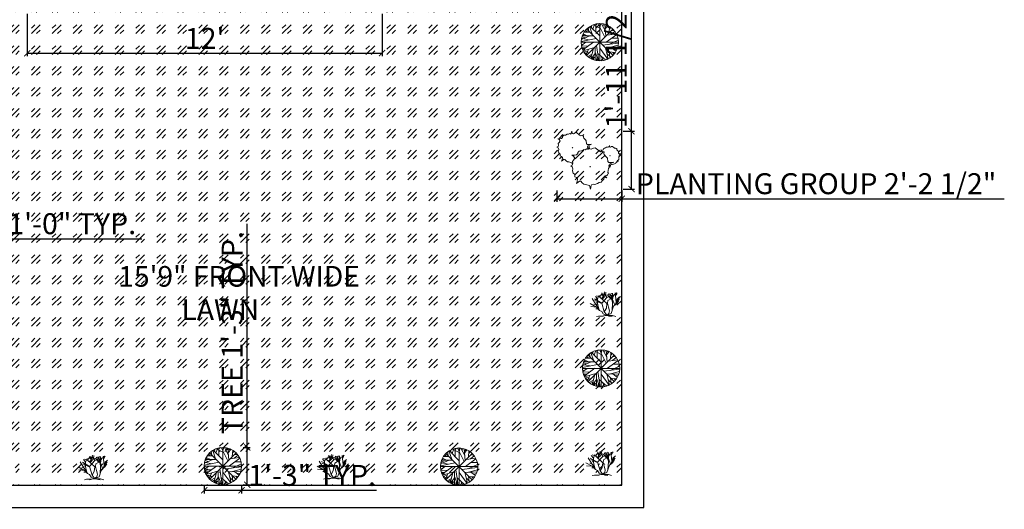
# Model space of a CAD drawing. Units: inches. Extents: x 3799 to 20199, y 1682 to 8087.
# Tile 8 of 30: x 11366 to 11765, y 2123 to 2322. Entities that reach past the tile are written whole.
import ezdxf

# ---------------------------------------------------------------- set-up
doc = ezdxf.new("R2010")
doc.units = ezdxf.units.IN
for name, color, linetype, lineweight in [('A-ANNO-DIMS', 2, 'Continuous', 18), ('A-ANNO-TEXT', 7, 'Continuous', 18), ('A-AREA-IDEN', 7, 'Continuous', 18), ('C-PROP', 7, 'Continuous', 25), ('L-PLNT', 94, 'Continuous', 13), ('L-PLNT-PATT', 94, 'Continuous', 13)]:
    doc.layers.add(name, color=color, linetype=linetype, lineweight=lineweight)
doc.styles.get("Standard").update_dxf_attribs({"font": 'arial.ttf'})
doc.dimstyles.new('ISO-25', dxfattribs={"dimtxt": 8.5, "dimasz": 2.5, "dimexe": 1.25, "dimexo": 0.625, "dimtad": 1, "dimdec": 0, "dimlunit": 3, "dimtxsty": 'Standard', "dimblk": 'ARCHTICK', "dimcen": 2.5, "dimadec": 0, "dimazin": 0, "dimtfac": 1, "dimtdec": 0, "dimtmove": 0, "dimatfit": 3, "dimfxl": 1, "dimarcsym": 0})

# ---------------------------------------------------------------- blocks, each defined once
blk = doc.blocks.new('Clump of Trees or Bushes - plan')
for points in [[(-10.993, 56.487), (-9.228, 58.426), (-10.144, 63.512), (-8.923, 67.033), (-3.43, 69.772), (2.673, 72.119), (-2.82, 71.728), (-10.449, 71.728), (-13.195, 74.075), (-13.806, 83.073), (-16.857, 86.594), (-22.045, 92.071), (-22.961, 94.81), (-22.656, 98.722), (-28.759, 100.678), (-31.811, 99.113), (-35.472, 101.461), (-45.543, 109.676), (-49.815, 108.503), (-55.308, 106.155), (-59.58, 106.938), (-60.801, 113.98), (-63.242, 104.982), (-67.209, 106.938), (-70.872, 104.59), (-74.839, 104.982), (-80.637, 101.461), (-86.435, 101.069), (-90.402, 97.548), (-90.402, 94.419), (-93.454, 90.898), (-98.947, 90.115), (-105.66, 90.115), (-101.083, 87.768), (-98.031, 82.682), (-100.778, 77.596), (-103.829, 74.466), (-103.219, 69.772), (-104.134, 65.077), (-108.102, 62.73), (-104.439, 60.774), (-102.609, 55.297), (-103.829, 50.211), (-102.303, 44.342), (-98.947, 41.995), (-98.031, 38.865), (-98.031, 34.953), (-93.148, 32.606), (-90.707, 29.476), (-91.317, 22.434), (-93.454, 17.348), (-89.487, 21.26), (-85.519, 23.999), (-82.468, 23.216), (-78.806, 19.304), (-74.228, 15.783), (-69.956, 15.392), (-59.886, 12.653), (-58.254, 7.074)], [(59.448, 5.262), (60.936, 4.858), (62.652, -1.011), (63.415, 4.858), (64.178, 5.836), (66.848, 6.814), (69.709, 6.569), (73.905, 7.792), (76.385, 9.748), (79.627, 10.237), (81.153, 12.438), (84.014, 15.127), (84.205, 17.084), (85.158, 17.573), (88.591, 16.839), (85.73, 20.262), (88.591, 20.751), (89.545, 21.974), (90.689, 24.174), (91.452, 24.663), (90.499, 25.886), (91.261, 31.999), (92.596, 33.466), (92.024, 36.645), (92.787, 38.845), (96.22, 40.557), (100.035, 42.024), (96.602, 41.779), (91.834, 41.779), (90.117, 43.246), (89.736, 48.871), (87.828, 51.071), (84.586, 54.494), (84.014, 56.206), (84.205, 58.651), (80.39, 59.873), (78.483, 58.895), (76.194, 60.362), (69.9, 65.497), (67.23, 64.764), (63.797, 63.297), (61.126, 63.786), (60.364, 68.187), (58.838, 62.563), (56.358, 63.786), (54.07, 62.319), (51.59, 62.563), (47.966, 60.362), (44.343, 60.118), (41.863, 57.917), (41.863, 55.961), (39.956, 53.761), (36.523, 53.272), (32.327, 53.272), (35.187, 51.805), (36.641, 49.381)]]:
    blk.add_lwpolyline(points)
for points in [[(-4.577, 66.508), (-7.629, 55.261), (-12.588, 57.706), (-17.166, 54.772), (-22.125, 55.261), (-29.372, 50.86), (-36.62, 50.371), (-41.579, 45.969), (-41.579, 42.057), (-45.393, 37.656), (-52.259, 36.678), (-60.651, 36.678), (-54.93, 33.743), (-51.115, 27.386), (-54.548, 21.029), (-58.363, 17.116), (-57.6, 11.248), (-58.744, 5.38), (-63.703, 2.446), (-59.126, 0), (-56.837, -6.846), (-58.363, -13.203), (-56.455, -20.539), (-52.259, -23.473), (-51.115, -27.385), (-51.115, -32.275), (-45.012, -35.21), (-41.96, -39.122), (-42.723, -47.924), (-45.393, -54.282), (-40.434, -49.391), (-35.475, -45.968), (-31.661, -46.946), (-27.083, -51.837), (-21.362, -56.238), (-16.021, -56.727), (-3.433, -60.15), (0, -71.887), (1.526, -60.15), (3.052, -58.194), (8.392, -56.238), (14.114, -56.727), (22.506, -54.282), (27.465, -50.369), (33.949, -49.391), (37.001, -44.99), (42.723, -39.611), (43.104, -35.699), (45.012, -34.721), (51.878, -36.188), (46.156, -29.341), (51.878, -28.363), (53.785, -25.918), (56.074, -21.517), (57.6, -20.539), (55.692, -18.094), (57.218, -5.868), (59.888, -2.934), (58.744, 3.424), (60.27, 7.825), (67.136, 11.248), (74.765, 14.182), (67.899, 13.693), (58.363, 13.693), (54.93, 16.627), (54.167, 27.875), (50.352, 32.276), (43.867, 39.123), (42.723, 42.546), (43.104, 47.436), (35.475, 49.882), (31.661, 47.925), (27.083, 50.86), (14.495, 61.129), (9.155, 59.662), (2.289, 56.728), (-3.052, 57.706)], [(-58.055, 61.947), (-58.97, 60.774), (-57.139, 60.774)], [(62.08, 35.667), (61.508, 34.933), (62.652, 34.933)], [(-1.144, 1.468), (-2.289, 0), (0, 0)]]:
    blk.add_lwpolyline(points, close=True)
blk = doc.blocks.new('Tree - deciduous plan')
for p, q in [((-49.8627, 32.8214), (-32.7853, 32.8214)), ((-45.8134, 38.2383), (-40.5318, 33.0471)), ((-43.8768, 36.4326), (-44.405, 40.2696)), ((42, 42), (-42, -42)), ((42, -42), (-42, 42)), ((-40.1797, 44.558), (-36.4825, 43.2038)), ((-37.0107, 47.0408), (-35.25, 35.5298)), ((-32.6092, 50.4264), (-23.2782, 23.5674)), ((-31.2008, 51.1035), (-0.2149, 20.1818)), ((-26.4472, 46.5894), (-26.2712, 53.8116)), ((-22.0458, 42.0753), (-16.5881, 57.6486)), ((-21.1656, 55.8436), (-0.0388, 45.0094)), ((-12.5388, 54.9406), (-7.9613, 59.4546)), ((-12.3627, 32.1443), (-12.5388, 58.7776)), ((-5.3205, 59.6806), (16.5105, 16.7963)), ((2.426, 54.9406), (-1.4472, 59.9056)), ((0, 59.9996), (0, -60)), ((0.4894, 48.6208), (3.6584, 59.6806)), ((18.2711, 35.5298), (5.419, 59.6806)), ((9.8203, 51.5549), (12.8133, 58.5516)), ((19.6795, 19.5047), (16.3344, 57.6486)), ((17.0387, 51.1035), (23.2006, 55.1666)), ((17.7429, 43.6552), (25.4894, 54.2636)), ((31.6513, 50.8778), (30.2429, 30.5643)), ((31.1232, 42.5267), (35.8767, 48.1693)), ((36.2288, 25.1474), (48.9049, 35.0784)), ((37.1091, 37.1098), (46.6161, 37.5612)), ((-59.7219, 2.8025), (-12.0106, 12.0565)), ((-32.2571, 20.6333), (-59.1937, 9.348)), ((-58.6656, 12.7336), (-35.9543, 7.5424)), ((-57.081, 17.9248), (-47.0458, 14.7649)), ((-56.0247, 20.859), (-20.8134, 20.859)), ((-54.7923, 24.4702), (-47.75, 21.0847)), ((-54.6162, -24.7335), (-20.2853, 0.0941)), ((-53.2078, 27.4044), (-40.1797, 20.859)), ((54.3626, 25.3731), (20.9119, 0.3198)), ((23.3767, 23.3417), (53.3063, 27.4044)), ((29.3626, -6.6771), (59.4682, 7.091)), ((38.5175, 13.4107), (58.2359, 13.6364)), ((-60, 0), (60, 0)), ((-59.7219, -4.8714), (-54.2641, -6.6771)), ((-45.2853, -0.1316), (-59.0177, -10.0627)), ((-58.4895, -12.3197), (-36.4825, -11.6426)), ((-57.081, -18.4138), (-45.2853, -17.9624)), ((-52.6797, -18.188), (-55.4966, -22.0251)), ((-53.2078, -27.442), (-16.7641, -16.6081)), ((-38.9472, -29.0219), (-51.4472, -30.6018)), ((-47.2219, -19.3166), (-50.2148, -26.3135)), ((-46.5177, -30.1504), (-49.5106, -33.536)), ((-35.9543, -22.4765), (-44.0529, -40.5329)), ((-19.9331, -20.2194), (-28.5599, -52.721)), ((-14.8275, -15.0282), (-14.6515, -57.6865)), ((-10.074, -10.0627), (-2.5036, -59.7178)), ((-0.0388, -19.0909), (25.8415, -53.8495)), ((9.2922, -9.1598), (59.6443, -2.8401)), ((18.6232, -18.6394), (26.7218, -53.3981)), ((18.7992, -18.6394), (57.3556, -17.2853)), ((26.3697, -18.4138), (58.9401, -9.8369)), ((30.419, -30.1504), (32.3556, -50.0125)), ((31.4753, -31.279), (49.6091, -33.3103)), ((38.1654, -18.188), (52.426, -29.0219)), ((45.9119, -24.0564), (55.595, -22.2508)), ((-32.4331, -32.4075), (-48.1021, -35.5674)), ((-43.7008, -34.6645), (-46.6937, -37.373)), ((-24.6867, -37.8244), (-38.7712, -45.7241)), ((-26.2712, -43.9185), (-34.7219, -48.6583)), ((-14.6515, -36.2445), (-27.6797, -52.9467)), ((-14.6515, -47.3041), (-25.0388, -54.3009)), ((-21.5177, -45.4984), (-19.9331, -56.1065)), ((-14.6515, -32.1818), (-3.912, -59.4922)), ((-8.4895, -47.5298), (-11.4825, -58.5893)), ((-6.3768, -52.721), (-9.3698, -58.815)), ((-6.2008, -36.2445), (17.919, -57.0094)), ((8.4119, -53.1724), (3.8344, -59.4922)), ((5.9471, -46.6269), (10.5246, -58.5893)), ((22.8485, -36.4702), (35.3485, -48.4326)), ((24.7852, -44.8213), (23.0246, -54.978)), ((41.5105, -32.6332), (46.088, -38.0501))]:
    blk.add_line(p, q)
blk.add_circle((0, 0), 60)
blk = doc.blocks.new('Shrub - elevation')
for p, q in [((-16.8, 16.32), (-18.72, 18.72)), ((-14.88, 18.24), (-17.76, 19.2)), ((-16.8, 16.32), (-15.36, 19.68)), ((-14.88, 18.24), (-12.96, 20.64)), ((-8.16, 12), (-14.88, 18.24)), ((-13.325, 16.724), (-11.433, 18.289)), ((-12.471, 19.775), (-12.898, 22.044)), ((-11.677, 19.071), (-12.471, 19.775)), ((-11.28, 19.619), (-12.104, 21.184)), ((-12.043, 15.628), (-11.921, 18.836)), ((-11.921, 18.836), (-10.64, 20.401)), ((-11.433, 18.289), (-10.457, 22.749)), ((-10.579, 18.054), (-9.846, 19.697)), ((-8.16, 17.76), (-10.56, 21.6)), ((-9.48, 19.775), (-8.992, 22.592)), ((-7.2, 19.68), (-8.64, 20.16)), ((-8.16, 17.76), (-5.28, 19.2)), ((-7.2, 19.68), (-6.24, 21.12)), ((-4.8, 16.32), (-7.2, 19.68)), ((-5.086, 17.741), (-5.513, 21.34)), ((-5.28, 19.2), (-3.84, 21.6)), ((-2.88, 12.96), (-4.32, 19.68)), ((-3.84, 16.8), (-0.96, 20.64)), ((-3.377, 18.602), (-2.888, 21.575)), ((-2.766, 16.802), (-3.377, 18.602)), ((-2.88, 15.84), (-2.4, 20.16)), ((-0.508, 21.888), (-0.081, 20.558)), ((-0.203, 19.149), (0.102, 21.34)), ((0.346, 13.203), (-0.203, 19.149)), ((-0.142, 19.384), (0.59, 20.401)), ((-0.02, 20.01), (0.896, 21.105)), ((0.041, 20.714), (1.384, 22.044)), ((0.102, 21.34), (0.835, 21.888)), ((1.323, 16.254), (3.642, 18.289)), ((-17.76, 8.64), (-23.663, 11.961)), ((-17.76, 8.64), (-23.128, 9.222)), ((-18.24, 11.04), (-21.755, 16.655)), ((-18.24, 11.04), (-20.16, 11.52)), ((-12.96, 12.48), (-19.68, 16.32)), ((-13.92, 12.48), (-19.2, 14.88)), ((-15.84, 8.16), (-18.24, 11.04)), ((-16.8, 12.48), (-17.76, 12.96)), ((-16.8, 12.48), (-16.8, 16.32)), ((-15.84, 8.16), (-16.8, 12.48)), ((-12.96, 12.48), (-13.92, 12.48)), ((-12.96, 12.48), (-8.16, 17.76)), ((-10.56, 4.32), (-12.96, 12.48)), ((-11.982, 16.802), (-10.579, 18.054)), ((-8.64, 7.68), (-8.16, 12)), ((-7.68, 12.48), (-7.2, 14.88)), ((-6.72, 8.64), (-7.68, 12.48)), ((-7.2, 14.88), (-3.84, 16.8)), ((-3.377, 15.315), (-5.086, 17.819)), ((-4.32, 2.88), (-1.92, 9.6)), ((-3.36, 5.28), (-2.88, 12.96)), ((-0.96, 10.56), (-2.88, 15.84)), ((-1.92, 9.6), (0.96, 12)), ((-0.48, 10.8), (0.346, 13.203)), ((0.346, 13.203), (1.323, 16.254)), ((0.96, 12), (1.44, 15.36)), ((0.96, 12), (2.88, 14.88)), ((1.44, 15.36), (2.88, 17.28)), ((1.92, 13.44), (2.4, 15.36)), ((2.4, 15.36), (3.36, 16.32)), ((-16.32, 7.2), (-18.24, 7.2)), ((-14.88, 5.76), (-17.76, 8.64)), ((-15.84, 0.48), (-17.76, 0)), ((-14.88, 5.76), (-15.84, 8.16)), ((-13.44, 0.48), (-15.84, 0.48)), ((-12.96, 4.8), (-14.88, 5.76)), ((-9.6, 0.96), (-13.44, 0.48)), ((-11.52, 2.4), (-12.96, 4.8)), ((-9.6, 0.96), (-12.96, 0)), ((-8.64, 0.96), (-11.52, 2.4)), ((-10.56, 4.32), (-8.64, 7.68)), ((-8.64, 1.92), (-10.56, 4.32)), ((-9.6, 0.96), (-7.68, 0.96)), ((-8.64, 0.96), (-4.32, 2.88)), ((-8.64, 0.96), (-6.24, 2.88)), ((-8.64, 0.96), (-8.64, 1.92)), ((-8.64, 0.96), (-2.88, 0.96)), ((-7.68, 0.96), (-6.24, 0.48)), ((-5.76, 5.28), (-6.72, 8.64)), ((-6.24, 2.88), (-5.76, 5.28)), ((-6.24, 0.48), (-3.36, 0)), ((-2.88, 0.96), (0, 0))]:
    blk.add_line(p, q)
blk = doc.blocks.new('_ArchTick')
at = {"color": 0, "linetype": 'ByBlock', "const_width": 0.15}
blk.add_lwpolyline([(-0.5, -0.5), (0.5, 0.5)], dxfattribs=at)
blk = doc.blocks.new('*D71')
at = {"layer": 'A-ANNO-DIMS', "color": 0, "lineweight": -2, "transparency": 16777216}
for p, q in [((11368.59, 2324.45), (11368.59, 2307.25)), ((11512.59, 2324.45), (11512.59, 2307.25)), ((11368.59, 2308.5), (11512.59, 2308.5))]:
    blk.add_line(p, q, dxfattribs=at)
at = {"layer": 'Defpoints', "color": 0, "transparency": 16777216}
for p in [(11368.59, 2325.07), (11512.59, 2325.07), (11512.59, 2308.5)]:
    blk.add_point(p, dxfattribs=at)
at = {"layer": 'A-ANNO-DIMS', "color": 0, "lineweight": -2, "transparency": 16777216, "xscale": 2.5, "yscale": 2.5, "zscale": 2.5, "rotation": 180}
blk.add_blockref('_ArchTick', (11368.59, 2308.5), dxfattribs=at)
at = {"layer": 'A-ANNO-DIMS', "color": 0, "lineweight": -2, "transparency": 16777216, "xscale": 2.5, "yscale": 2.5, "zscale": 2.5}
blk.add_blockref('_ArchTick', (11512.59, 2308.5), dxfattribs=at)
at = {"layer": 'A-ANNO-DIMS', "color": 0, "transparency": 16777216, "insert": (11440.59, 2313.39), "char_height": 8.5, "attachment_point": 5}
blk.add_mtext("12'", dxfattribs=at)
blk = doc.blocks.new('*D286')
at = {"layer": 'A-ANNO-DIMS', "color": 0, "lineweight": -2, "transparency": 16777216}
for p, q in [((11457.82, 2148.45), (11457.82, 2239.19)), ((11456.17, 2148.45), (11459.07, 2148.45)), ((11457.82, 2133.3), (11457.82, 2148.45)), ((11456.17, 2133.3), (11459.07, 2133.3))]:
    blk.add_line(p, q, dxfattribs=at)
at = {"layer": 'Defpoints', "color": 0, "transparency": 16777216}
for p in [(11455.55, 2148.45), (11457.82, 2148.45), (11455.55, 2133.3)]:
    blk.add_point(p, dxfattribs=at)
at = {"layer": 'A-ANNO-DIMS', "color": 0, "lineweight": -2, "transparency": 16777216, "xscale": 2.5, "yscale": 2.5, "zscale": 2.5}
for p, rotation in [((11457.82, 2148.45), 90), ((11457.82, 2133.3), 270)]:
    blk.add_blockref('_ArchTick', p, dxfattribs=dict(at, rotation=rotation))
at = {"layer": 'A-ANNO-DIMS', "color": 0, "transparency": 16777216, "insert": (11452.85, 2195.07), "char_height": 8.5, "attachment_point": 5, "rotation": 90}
blk.add_mtext('TREE 1\'-3" TYP.', dxfattribs=at)
blk = doc.blocks.new('*D287')
at = {"layer": 'A-ANNO-DIMS', "color": 0, "lineweight": -2, "transparency": 16777216}
for p, q in [((11440.4, 2132.67), (11440.4, 2129.78)), ((11440.4, 2131.03), (11455.55, 2131.03)), ((11455.55, 2132.67), (11455.55, 2129.78)), ((11455.55, 2131.03), (11510.31, 2131.03))]:
    blk.add_line(p, q, dxfattribs=at)
at = {"layer": 'Defpoints', "color": 0, "transparency": 16777216}
for p in [(11440.4, 2133.3), (11455.55, 2133.3), (11455.55, 2131.03)]:
    blk.add_point(p, dxfattribs=at)
at = {"layer": 'A-ANNO-DIMS', "color": 0, "lineweight": -2, "transparency": 16777216, "xscale": 2.5, "yscale": 2.5, "zscale": 2.5, "rotation": 180}
blk.add_blockref('_ArchTick', (11440.4, 2131.03), dxfattribs=at)
at = {"layer": 'A-ANNO-DIMS', "color": 0, "lineweight": -2, "transparency": 16777216, "xscale": 2.5, "yscale": 2.5, "zscale": 2.5}
blk.add_blockref('_ArchTick', (11455.55, 2131.03), dxfattribs=at)
at = {"layer": 'A-ANNO-DIMS', "color": 0, "transparency": 16777216, "insert": (11484.18, 2135.99), "char_height": 8.5, "attachment_point": 5}
blk.add_mtext('1\'-3" TYP.', dxfattribs=at)
blk = doc.blocks.new('*D300')
at = {"layer": 'A-ANNO-DIMS', "color": 0, "lineweight": -2, "transparency": 16777216}
for p, q in [((11302.78, 2234.32), (11302.78, 2231.9)), ((11314.75, 2234.32), (11314.75, 2231.9)), ((11302.78, 2233.15), (11314.75, 2233.15)), ((11314.75, 2233.15), (11415.14, 2233.15))]:
    blk.add_line(p, q, dxfattribs=at)
at = {"layer": 'Defpoints', "color": 0, "transparency": 16777216}
for p in [(11302.78, 2234.95), (11314.75, 2234.95), (11314.75, 2233.15)]:
    blk.add_point(p, dxfattribs=at)
at = {"layer": 'A-ANNO-DIMS', "color": 0, "lineweight": -2, "transparency": 16777216, "xscale": 2.5, "yscale": 2.5, "zscale": 2.5, "rotation": 180}
blk.add_blockref('_ArchTick', (11302.78, 2233.15), dxfattribs=at)
at = {"layer": 'A-ANNO-DIMS', "color": 0, "lineweight": -2, "transparency": 16777216, "xscale": 2.5, "yscale": 2.5, "zscale": 2.5}
blk.add_blockref('_ArchTick', (11314.75, 2233.15), dxfattribs=at)
at = {"layer": 'A-ANNO-DIMS', "color": 0, "transparency": 16777216, "insert": (11366.2, 2238.17), "char_height": 8.5, "attachment_point": 5}
blk.add_mtext('SHRUB 1\'-0" TYP.', dxfattribs=at)
blk = doc.blocks.new('*D348')
at = {"layer": 'A-ANNO-DIMS', "color": 0, "lineweight": -2, "transparency": 16777216}
for p, q in [((11583.56, 2252.71), (11583.56, 2248.14)), ((11609.84, 2252.71), (11609.84, 2248.14)), ((11583.56, 2249.39), (11609.84, 2249.39)), ((11609.84, 2249.39), (11765.09, 2249.39))]:
    blk.add_line(p, q, dxfattribs=at)
at = {"layer": 'Defpoints', "color": 0, "transparency": 16777216}
for p in [(11583.56, 2253.33), (11609.84, 2253.33), (11609.84, 2249.39)]:
    blk.add_point(p, dxfattribs=at)
at = {"layer": 'A-ANNO-DIMS', "color": 0, "lineweight": -2, "transparency": 16777216, "xscale": 2.5, "yscale": 2.5, "zscale": 2.5, "rotation": 180}
blk.add_blockref('_ArchTick', (11583.56, 2249.39), dxfattribs=at)
at = {"layer": 'A-ANNO-DIMS', "color": 0, "lineweight": -2, "transparency": 16777216, "xscale": 2.5, "yscale": 2.5, "zscale": 2.5}
blk.add_blockref('_ArchTick', (11609.84, 2249.39), dxfattribs=at)
at = {"layer": 'A-ANNO-DIMS', "color": 0, "transparency": 16777216, "insert": (11688.72, 2254.41), "char_height": 8.5, "attachment_point": 5}
blk.add_mtext('PLANTING GROUP 2\'-2 1/2"', dxfattribs=at)
blk = doc.blocks.new('*D349')
at = {"layer": 'A-ANNO-DIMS', "color": 0, "lineweight": -2, "transparency": 16777216}
for p, q in [((11613.78, 2276.8), (11613.78, 2328.76)), ((11610.46, 2276.8), (11615.03, 2276.8)), ((11613.78, 2253.33), (11613.78, 2276.8)), ((11610.46, 2253.33), (11615.03, 2253.33))]:
    blk.add_line(p, q, dxfattribs=at)
at = {"layer": 'Defpoints', "color": 0, "transparency": 16777216}
for p in [(11609.84, 2276.8), (11613.78, 2276.8), (11609.84, 2253.33)]:
    blk.add_point(p, dxfattribs=at)
at = {"layer": 'A-ANNO-DIMS', "color": 0, "lineweight": -2, "transparency": 16777216, "xscale": 2.5, "yscale": 2.5, "zscale": 2.5}
for p, rotation in [((11613.78, 2276.8), 90), ((11613.78, 2253.33), 270)]:
    blk.add_blockref('_ArchTick', p, dxfattribs=dict(at, rotation=rotation))
at = {"layer": 'A-ANNO-DIMS', "color": 0, "transparency": 16777216, "insert": (11608.76, 2304.03), "char_height": 8.5, "attachment_point": 5, "rotation": 90}
blk.add_mtext('1\'-11 1/2"', dxfattribs=at)

msp = doc.modelspace()

# ---------------------------------------------------------------- hatches: boundary and pattern name
at = {"layer": 'L-PLNT-PATT'}
h = msp.add_hatch(dxfattribs=at)
h.set_pattern_fill('GOST_GLASS', color=256)
h.paths.add_polyline_path([(11609.85, 2325.07), (11549.85, 2325.07), (11315.85, 2325.07), (11315.85, 2300.82), (11302.02, 2300.82), (11302.02, 2133.07), (11609.85, 2133.07)])
h.paths.add_polyline_path([(11496.55, 2144.31), (11496.62, 2144.39), (11496.58, 2144.52)], flags=16)
h.paths.add_polyline_path([(11491.91, 2145.12), (11493.01, 2143.36), (11494.28, 2143.99), (11494.28, 2144.01), (11494.36, 2143.39), (11494.73, 2142.84), (11494.91, 2142.94), (11495.46, 2143.67), (11495.33, 2142.52), (11496.19, 2140.15), (11495.75, 2139.78), (11494.7, 2136.83), (11492.98, 2136.07), (11493.22, 2135.99), (11492.8, 2135.99), (11491.54, 2136.62), (11490.91, 2137.68), (11490.07, 2138.1), (11489.64, 2139.15), (11489.22, 2141.04), (11489.22, 2142.73), (11489.64, 2143.71), (11490.07, 2143.57), (11491.02, 2144.77), (11491.12, 2144.24), (11491.46, 2143.95), (11491.73, 2144.28)], flags=16)
h.paths.add_polyline_path([(11491.31, 2142.42), (11493.01, 2140.83), (11492.8, 2138.94), (11491.96, 2137.47), (11490.91, 2141.04), (11491.77, 2141.99), (11490.77, 2142.92), (11491.35, 2143.4)], flags=0)
h.paths.add_polyline_path([(11455.55, 2140.87), (11453.52, 2140.87), (11451.69, 2140.04), (11455.54, 2140.52, 0.011687)], flags=16)
h.paths.add_polyline_path([(11451.82, 2137.03), (11451.82, 2136.94), (11451.92, 2136.93)], flags=16)
h.paths.add_polyline_path([(11447.97, 2140.87), (11447.97, 2135.62), (11447.21, 2136.28), (11446.7, 2139.6), (11446.1, 2139), (11446.11, 2136.84), (11446.26, 2136.47), (11446.11, 2136.28), (11446.12, 2134.9), (11445.36, 2134.39), (11445.25, 2135.18), (11446.11, 2136.28), (11446.1, 2138.85), (11445.88, 2138.78), (11443.88, 2136.78), (11442.77, 2136.56), (11443.44, 2138.06), (11441.62, 2137.52), (11442.08, 2138.6), (11442.26, 2138.61), (11442, 2138.42), (11441.62, 2137.52), (11445.88, 2138.78), (11447.97, 2140.87), (11447.97, 2143.39), (11445.18, 2146.18), (11445.72, 2147.71), (11447.97, 2146.55), (11447.97, 2148.2), (11448.27, 2147.82), (11448.02, 2146.98), (11450.07, 2142.97)], flags=16)
h.paths.add_polyline_path([(11551.41, 2140.65, -1), (11536.26, 2140.65, -1)])
h.paths.add_polyline_path([(11547.68, 2136.8), (11547.69, 2136.71), (11547.78, 2136.7)], flags=16)
h.paths.add_polyline_path([(11541.05, 2145.95), (11541.58, 2147.48), (11542.26, 2147.14), (11542.27, 2144.73)], flags=16)
h.paths.add_polyline_path([(11541.96, 2138.78), (11541.97, 2136.62), (11542.12, 2136.24), (11541.97, 2136.06), (11541.98, 2134.67), (11541.23, 2134.17), (11541.11, 2134.95), (11541.97, 2136.06), (11541.96, 2138.62), (11541.74, 2138.56), (11539.74, 2136.56), (11538.63, 2136.33), (11539.3, 2137.83), (11537.48, 2137.29), (11537.94, 2138.37), (11538.12, 2138.38), (11541.25, 2140.65), (11543.83, 2140.65)], flags=16)
h.paths.add_polyline_path([(11584.29, 2268.01), (11584.1, 2268.75), (11584.25, 2269.39), (11584.02, 2270.08), (11583.56, 2270.33), (11584.06, 2270.63), (11584.18, 2271.22), (11584.1, 2271.81), (11584.48, 2272.21), (11584.83, 2272.85), (11584.45, 2273.49), (11583.87, 2273.79), (11584.72, 2273.79), (11585.41, 2273.89), (11585.79, 2274.33), (11585.79, 2274.73), (11586.3, 2275.17), (11587.03, 2275.22), (11587.76, 2275.66), (11588.26, 2275.62), (11588.72, 2275.91), (11589.22, 2275.66), (11589.53, 2276.8), (11589.69, 2275.91), (11590.23, 2275.81), (11590.92, 2276.11), (11591.46, 2276.26), (11592.73, 2275.22), (11593.19, 2274.92), (11593.58, 2275.12), (11594.35, 2274.87), (11594.31, 2274.38), (11594.43, 2274.03), (11595.08, 2273.34), (11595.47, 2272.9), (11595.54, 2271.76), (11595.89, 2271.47), (11596.85, 2271.47), (11597.55, 2271.52), (11596.78, 2271.22), (11596.08, 2270.87), (11595.93, 2270.43), (11596.04, 2269.79), (11595.85, 2269.58), (11596.25, 2269.39), (11596.63, 2270.81), (11596.82, 2269.7), (11597.5, 2269.57), (11598.36, 2269.94), (11599.04, 2270.13), (11600.63, 2268.83), (11601.21, 2268.46), (11601.77, 2268.75), (11601.65, 2268.95), (11601.29, 2269.14), (11601.82, 2269.14), (11602.25, 2269.2), (11602.49, 2269.48), (11602.49, 2269.72), (11602.81, 2270), (11603.26, 2270.03), (11603.72, 2270.31), (11604.04, 2270.28), (11604.32, 2270.46), (11604.64, 2270.31), (11604.83, 2271.02), (11604.93, 2270.46), (11605.26, 2270.4), (11605.7, 2270.59), (11606.03, 2270.68), (11606.83, 2270.03), (11607.12, 2269.85), (11607.36, 2269.97), (11607.84, 2269.82), (11607.82, 2269.51), (11607.89, 2269.29), (11608.3, 2268.86), (11608.54, 2268.58), (11608.59, 2267.87), (11608.8, 2267.68), (11609.4, 2267.68), (11609.84, 2267.72), (11609.36, 2267.53), (11608.92, 2267.31), (11608.83, 2267.04), (11608.9, 2266.64), (11608.73, 2266.45), (11608.63, 2265.68), (11608.75, 2265.52), (11608.66, 2265.46), (11608.44, 2265.04), (11608.03, 2264.97), (11608.39, 2264.54), (11607.96, 2264.63), (11607.84, 2264.57), (11607.82, 2264.32), (11607.45, 2263.98), (11607.26, 2263.7), (11606.85, 2263.64), (11606.54, 2263.39), (11606.01, 2263.24), (11605.65, 2263.27), (11605.31, 2263.15), (11605.21, 2263.02), (11605.12, 2262.28), (11604.9, 2263.02), (11604.71, 2263.08), (11604.63, 2262.84), (11604.77, 2262.04), (11604.43, 2261.67), (11604.24, 2260.13), (11604.48, 2259.82), (11604.29, 2259.69), (11604, 2259.14), (11603.76, 2258.83), (11603.04, 2258.71), (11603.76, 2257.84), (11602.89, 2258.03), (11602.65, 2257.9), (11602.6, 2257.41), (11601.88, 2256.73), (11601.49, 2256.17), (11600.68, 2256.05), (11600.05, 2255.56), (11598.99, 2255.25), (11598.27, 2255.31), (11597.59, 2255.06), (11597.4, 2254.82), (11597.21, 2253.33), (11596.77, 2254.82), (11595.19, 2255.25), (11594.51, 2255.31), (11593.79, 2255.87), (11593.21, 2256.48), (11592.73, 2256.61), (11592.1, 2256.17), (11591.48, 2255.56), (11591.81, 2256.36), (11591.91, 2257.47), (11591.53, 2257.96), (11590.75, 2258.34), (11590.75, 2258.95), (11590.61, 2259.45), (11590.08, 2259.82), (11589.84, 2260.74), (11590.03, 2261.55), (11589.74, 2262.41), (11589.17, 2262.72), (11589.79, 2263.09), (11589.84, 2263.34), (11589.65, 2264.01), (11588.38, 2264.35), (11587.84, 2264.4), (11587.26, 2264.85), (11586.8, 2265.34), (11586.41, 2265.44), (11585.91, 2265.09), (11585.41, 2264.6), (11585.68, 2265.24), (11585.76, 2266.13), (11585.45, 2266.53), (11584.83, 2266.82), (11584.83, 2267.32), (11584.72, 2267.71)], flags=16)
h.paths.add_polyline_path([(11589.76, 2270.08), (11589.88, 2270.23), (11589.99, 2270.08)], flags=0)
h.paths.add_polyline_path([(11596.92, 2262.41), (11597.06, 2262.6), (11597.21, 2262.41)], flags=0)
h.paths.add_polyline_path([(11607.36, 2210.31), (11607.43, 2210.39), (11607.39, 2210.52)], flags=16)
h.paths.add_polyline_path([(11600.87, 2204.1), (11600.45, 2205.15), (11600.03, 2207.04), (11600.03, 2208.73), (11600.45, 2209.71), (11600.87, 2209.57), (11601.83, 2210.77), (11601.93, 2210.24), (11602.27, 2209.95), (11602.54, 2210.28), (11602.72, 2211.12), (11603.82, 2209.36), (11605.09, 2209.99), (11605.09, 2210), (11605.17, 2209.39), (11605.54, 2208.84), (11605.72, 2208.94), (11606.27, 2209.67), (11606.14, 2208.52), (11607, 2206.15), (11606.56, 2205.78), (11605.51, 2202.83), (11603.79, 2202.07), (11604.03, 2201.99), (11603.61, 2201.99), (11602.35, 2202.62), (11601.72, 2203.68)], flags=16)
h.paths.add_polyline_path([(11601.72, 2207.04), (11602.58, 2207.99), (11601.57, 2208.92), (11602.16, 2209.4), (11602.12, 2208.42), (11603.82, 2206.83), (11603.61, 2204.94), (11602.77, 2203.47)], flags=0)
h.paths.add_polyline_path([(11399.57, 2144.02), (11399.64, 2144.1), (11399.6, 2144.23)], flags=16)
h.paths.add_polyline_path([(11398.77, 2139.49), (11397.71, 2136.54), (11396, 2135.78), (11396.24, 2135.7), (11395.82, 2135.7), (11394.55, 2136.33), (11393.92, 2137.38), (11393.08, 2137.81), (11392.66, 2138.86), (11392.24, 2140.75), (11392.24, 2142.44), (11392.66, 2143.42), (11393.08, 2143.28), (11394.04, 2144.48), (11394.14, 2143.95), (11394.47, 2143.66), (11394.74, 2143.99), (11394.93, 2144.83), (11396.03, 2143.07), (11397.29, 2143.7), (11397.3, 2143.71), (11397.37, 2143.1), (11397.75, 2142.55), (11397.92, 2142.65), (11398.47, 2143.38), (11398.34, 2142.23), (11399.21, 2139.86)], flags=16)
h.paths.add_polyline_path([(11609.04, 2180.55, -1), (11593.89, 2180.55, -1)], flags=16)
h.paths.add_polyline_path([(11605.31, 2176.71), (11605.32, 2176.61), (11605.41, 2176.6)], flags=0)
h.paths.add_polyline_path([(11601.47, 2180.55), (11601.47, 2183.07), (11598.68, 2185.85), (11599.22, 2187.38), (11601.47, 2186.23), (11601.47, 2187.88), (11601.76, 2187.5), (11601.52, 2186.66), (11603.57, 2182.65), (11601.47, 2180.55), (11601.47, 2175.3), (11600.7, 2175.96), (11600.2, 2179.28), (11599.6, 2178.68), (11599.61, 2176.52), (11599.75, 2176.15), (11599.61, 2175.96), (11599.61, 2174.57), (11598.86, 2174.07), (11598.74, 2174.85), (11599.61, 2175.96), (11599.6, 2178.53), (11599.38, 2178.46), (11597.38, 2176.46), (11596.27, 2176.23), (11596.94, 2177.74), (11595.11, 2177.19), (11595.58, 2178.28), (11595.76, 2178.28), (11598.89, 2180.55)], flags=0)
h.paths.add_polyline_path([(11394.33, 2142.12), (11396.03, 2140.54), (11395.82, 2138.65), (11394.98, 2137.17), (11393.92, 2140.75), (11394.78, 2141.7), (11393.78, 2142.63), (11394.36, 2143.11)], flags=0)
h.paths.add_polyline_path([(11604.97, 2266.82), (11605.05, 2266.91), (11605.12, 2266.82)], flags=0)
h.paths.add_polyline_path([(11593.36, 2312.93, -1), (11608.51, 2312.93, -1)], flags=16)
h.paths.add_polyline_path([(11604.78, 2309.09), (11604.79, 2309), (11604.88, 2308.99)], flags=0)
h.paths.add_polyline_path([(11596.4, 2310.12), (11594.58, 2309.58), (11595.04, 2310.66), (11595.22, 2310.66), (11598.35, 2312.93), (11600.93, 2312.93), (11600.93, 2315.45), (11598.15, 2318.23), (11598.68, 2319.77), (11600.93, 2318.61), (11600.93, 2320.26), (11601.23, 2319.88), (11600.99, 2319.04), (11603.03, 2315.03), (11600.93, 2312.93), (11600.93, 2307.68), (11600.17, 2308.34), (11599.66, 2311.66), (11599.06, 2311.06), (11599.07, 2308.9), (11599.22, 2308.53), (11599.07, 2308.34), (11599.08, 2306.96), (11598.33, 2306.45), (11598.21, 2307.24), (11599.07, 2308.34), (11599.06, 2310.91), (11598.84, 2310.84), (11596.84, 2308.84), (11595.73, 2308.62)], flags=0)
h.paths.add_polyline_path([(11605.66, 2145.72), (11605.73, 2145.8), (11605.69, 2145.93)], flags=16)
h.paths.add_polyline_path([(11598.75, 2140.56), (11598.33, 2142.46), (11598.33, 2144.14), (11598.75, 2145.12), (11599.17, 2144.98), (11600.13, 2146.18), (11600.23, 2145.66), (11600.56, 2145.36), (11600.83, 2145.69), (11601.02, 2146.53), (11602.12, 2144.77), (11603.38, 2145.4), (11603.39, 2145.42), (11603.46, 2144.81), (11603.84, 2144.25), (11604.02, 2144.35), (11604.56, 2145.08), (11604.44, 2143.93), (11605.3, 2141.56), (11604.86, 2141.19), (11603.8, 2138.25), (11602.09, 2137.48), (11602.33, 2137.4), (11601.91, 2137.4), (11600.65, 2138.04), (11600.01, 2139.09), (11599.17, 2139.51)], flags=16)
h.paths.add_polyline_path([(11600.01, 2142.46), (11600.87, 2143.4), (11599.87, 2144.33), (11600.45, 2144.81), (11600.42, 2143.83), (11602.12, 2142.25), (11601.91, 2140.35), (11601.07, 2138.88)], flags=0)
h.paths.add_polyline_path([(11363.83, 2141.59, -1), (11348.68, 2141.59, -1)], flags=0)
h.paths.add_polyline_path([(11360.1, 2137.75), (11360.11, 2137.66), (11360.2, 2137.65)], flags=0)
h.paths.add_polyline_path([(11356.26, 2141.59), (11356.26, 2136.34), (11355.49, 2137), (11354.98, 2140.32), (11354.38, 2139.72), (11354.39, 2137.56), (11354.54, 2137.19), (11354.39, 2137), (11354.4, 2135.62), (11353.65, 2135.11), (11353.53, 2135.9), (11354.39, 2137), (11354.38, 2139.57), (11354.17, 2139.5), (11352.16, 2137.5), (11351.05, 2137.28), (11351.73, 2138.78), (11349.9, 2138.24), (11350.36, 2139.32), (11350.54, 2139.33), (11353.68, 2141.59), (11356.26, 2141.59), (11356.26, 2144.11), (11353.47, 2146.9), (11354.01, 2148.43), (11356.26, 2147.27), (11356.26, 2148.92), (11356.55, 2148.54), (11356.31, 2147.7), (11358.35, 2143.69)], flags=0)
h.paths.add_polyline_path([(11313.11, 2243.68), (11313.18, 2243.77), (11313.14, 2243.89)], flags=16)
h.paths.add_polyline_path([(11312.31, 2239.16), (11311.26, 2236.21), (11309.55, 2235.45), (11309.79, 2235.37), (11309.37, 2235.37), (11308.1, 2236), (11307.47, 2237.05), (11306.63, 2237.47), (11306.21, 2238.53), (11305.79, 2240.42), (11305.79, 2242.11), (11306.21, 2243.09), (11306.63, 2242.95), (11307.59, 2244.15), (11307.68, 2243.62), (11308.02, 2243.32), (11308.29, 2243.65), (11308.47, 2244.5), (11309.58, 2242.74), (11310.84, 2243.37), (11310.85, 2243.38), (11310.92, 2242.77), (11311.3, 2242.22), (11311.47, 2242.32), (11312.02, 2243.05), (11311.89, 2241.9), (11312.75, 2239.53)], flags=16)
h.paths.add_polyline_path([(11308.52, 2236.84), (11307.47, 2240.42), (11308.33, 2241.37), (11307.33, 2242.3), (11307.91, 2242.78), (11307.87, 2241.79), (11309.58, 2240.21), (11309.37, 2238.32)], flags=0)
h.paths.add_polyline_path([(11302.02, 2281.94, -1), (11317.17, 2281.94, -1)])
h.paths.add_polyline_path([(11313.44, 2278.1), (11313.44, 2278), (11313.54, 2277.99)], flags=16)
h.paths.add_polyline_path([(11309.59, 2276.69), (11308.83, 2277.35), (11308.32, 2280.67), (11307.72, 2280.07), (11307.73, 2277.91), (11307.88, 2277.54), (11307.73, 2277.35), (11307.74, 2275.96), (11306.98, 2275.46), (11306.87, 2276.24), (11307.73, 2277.35), (11307.72, 2279.92), (11307.5, 2279.85), (11305.5, 2277.85), (11304.39, 2277.63), (11305.06, 2279.13), (11303.24, 2278.58), (11303.7, 2279.67), (11303.88, 2279.67), (11303.62, 2279.49), (11303.24, 2278.58), (11307.5, 2279.85), (11309.59, 2281.94), (11309.59, 2284.46), (11306.8, 2287.24), (11307.34, 2288.77), (11309.59, 2287.62), (11309.59, 2289.27), (11309.89, 2288.89), (11309.64, 2288.05), (11311.69, 2284.04), (11309.59, 2281.94)], flags=16)
h.paths.add_polyline_path([(11317.17, 2181.83, -1), (11302.02, 2181.83, -1)])
h.paths.add_polyline_path([(11313.44, 2177.98), (11313.44, 2177.89), (11313.54, 2177.88)], flags=16)
h.paths.add_polyline_path([(11309.59, 2181.83), (11309.59, 2176.58), (11308.83, 2177.24), (11308.32, 2180.56), (11307.72, 2179.96), (11307.73, 2177.8), (11307.88, 2177.42), (11307.73, 2177.24), (11307.74, 2175.85), (11306.98, 2175.35), (11306.87, 2176.13), (11307.73, 2177.24), (11307.72, 2179.8), (11307.5, 2179.74), (11305.5, 2177.74), (11304.39, 2177.51), (11305.06, 2179.01), (11303.24, 2178.47), (11303.7, 2179.55), (11303.88, 2179.56), (11303.62, 2179.38), (11303.24, 2178.47), (11307.5, 2179.74), (11309.59, 2181.83), (11309.59, 2184.35), (11306.8, 2187.13), (11307.34, 2188.66), (11309.59, 2187.51), (11309.59, 2189.16), (11309.89, 2188.78), (11309.64, 2187.94), (11311.69, 2183.93)], flags=16)
h.paths.add_polyline_path([(11318.27, 2141.81), (11318.34, 2141.89), (11318.3, 2142.02)], flags=16)
h.paths.add_polyline_path([(11317.47, 2137.28), (11316.41, 2134.34), (11314.7, 2133.57), (11314.94, 2133.49), (11314.52, 2133.49), (11313.26, 2134.12), (11312.62, 2135.18), (11311.78, 2135.6), (11311.36, 2136.65), (11310.94, 2138.55), (11310.94, 2140.23), (11311.36, 2141.21), (11311.78, 2141.07), (11312.74, 2142.27), (11312.84, 2141.75), (11313.17, 2141.45), (11313.44, 2141.78), (11313.63, 2142.62), (11314.73, 2140.86), (11315.99, 2141.49), (11316, 2141.51), (11316.07, 2140.9), (11316.45, 2140.34), (11316.62, 2140.44), (11317.17, 2141.17), (11317.05, 2140.02), (11317.91, 2137.65)], flags=16)
h.paths.add_polyline_path([(11314.73, 2138.34), (11314.52, 2136.44), (11313.68, 2134.97), (11312.62, 2138.55), (11313.48, 2139.49), (11312.48, 2140.42), (11313.06, 2140.9), (11313.03, 2139.92)], flags=0)
h.paths.add_polyline_path([(11454.71, 2144.33), (11450.92, 2143.82), (11447.97, 2140.87), (11455.55, 2140.87, 0.119183)], flags=16)
h.paths.add_polyline_path([(11450.07, 2142.97), (11448.02, 2146.98), (11447.97, 2147.09), (11447.97, 2146.55), (11447.97, 2140.87)], flags=0)
h.paths.add_polyline_path([(11447.97, 2143.39), (11445.18, 2146.18), (11445.72, 2147.71), (11445.88, 2148.15, 0.334379), (11440.4, 2140.87), (11447.97, 2140.87)], flags=0)
h.paths.add_polyline_path([(11447.97, 2143.39), (11447.97, 2146.55), (11447.97, 2148.45, 0.414214), (11440.4, 2140.87), (11447.97, 2140.87)], flags=16)
h.paths.add_polyline_path([(11447.97, 2138.46), (11447.97, 2135.62), (11447.97, 2133.3, 0.158969), (11452.44, 2134.75), (11450.84, 2136.28), (11451.1, 2135.2), (11450.97, 2134.44)], flags=16)
h.paths.add_polyline_path([(11348.68, 2141.59, 1), (11363.83, 2141.59, 1)], flags=16)
h.paths.add_polyline_path([(11360.1, 2137.75), (11360.28, 2135.9), (11359.13, 2137), (11358.61, 2139.24)], flags=0)
h.paths.add_polyline_path([(11362.99, 2145.05), (11359.2, 2144.54), (11356.26, 2141.59), (11361.81, 2141.59), (11363.78, 2142.49, 0.08904)], flags=0)
h = msp.add_hatch(dxfattribs=at)
h.set_pattern_fill('GOST_GLASS', color=256)
h.paths.add_polyline_path([(11363.12, 2144.8, 0.009445), (11362.99, 2145.05), (11359.2, 2144.54), (11356.26, 2141.59), (11361.81, 2141.59), (11363.78, 2142.49, 0.027518), (11363.63, 2143.31), (11361.1, 2143.29)])
h.paths.add_polyline_path([(11356.26, 2147.81), (11356.26, 2141.59), (11358.35, 2143.69)])
h.paths.add_polyline_path([(11315.78, 2135.39), (11315.36, 2136.86), (11314.94, 2138.55), (11315.15, 2139.6), (11316.22, 2140.21), (11315.48, 2141.24), (11314.73, 2140.86), (11313.48, 2139.49), (11314.73, 2138.34), (11314.52, 2136.44), (11313.68, 2134.97), (11314.52, 2133.91), (11314.52, 2133.49), (11315.57, 2134.34)])
h.paths.add_polyline_path([(11314.73, 2138.34), (11313.48, 2139.49), (11312.62, 2138.55), (11313.68, 2134.97), (11314.52, 2136.44)])
h.paths.add_polyline_path([(11317.05, 2138.76), (11316.82, 2139.8), (11316.45, 2140.34), (11315.15, 2139.6), (11314.94, 2138.55), (11315.36, 2136.86), (11315.78, 2135.39), (11315.57, 2134.34), (11314.52, 2133.49), (11316.41, 2134.34), (11316.84, 2135.54)])
h.paths.add_polyline_path([(11312.62, 2138.55), (11312.2, 2138.55), (11310.94, 2139.12), (11310.94, 2138.55), (11311.36, 2136.65), (11311.78, 2135.6), (11312.62, 2135.18), (11313.26, 2134.12), (11314.52, 2133.49), (11314.52, 2133.91), (11313.68, 2134.97)])
h.paths.add_polyline_path([(11313.48, 2139.49), (11311.78, 2141.07), (11311.36, 2141.21), (11310.94, 2140.23), (11310.94, 2139.51), (11312.62, 2138.55)])
h.paths.add_polyline_path([(11309.59, 2181.83), (11309.59, 2179.41), (11312.59, 2175.39), (11312.72, 2176.15), (11311.94, 2179.48)])
h.paths.add_polyline_path([(11309.59, 2181.83), (11307.01, 2181.83), (11302.69, 2178.7, 0.110902), (11304.69, 2176.05), (11306.49, 2177.06), (11305.98, 2175.17, 0.124716), (11309.59, 2174.25), (11309.59, 2176.58), (11308.83, 2177.24), (11308.32, 2180.56)])
h.paths.add_polyline_path([(11309.59, 2189.4), (11309.59, 2181.83), (11317.17, 2181.83, 0.414214)])
h.paths.add_polyline_path([(11309.59, 2189.4, 0.352911), (11302.19, 2183.44), (11302.8, 2183.29), (11302.11, 2183, 0.03899), (11302.02, 2181.83), (11309.59, 2181.83)])
h.paths.add_polyline_path([(11308.07, 2183.35), (11309.59, 2181.83), (11309.59, 2189.4, 0.352911), (11302.19, 2183.44), (11302.8, 2183.29), (11302.11, 2183, 0.03899), (11302.02, 2181.83), (11309.59, 2181.83)], flags=16)
h.paths.add_polyline_path([(11604.44, 2142.67), (11604.21, 2143.71), (11603.84, 2144.25), (11602.54, 2143.51), (11602.33, 2142.46), (11602.75, 2140.77), (11603.17, 2139.3), (11602.96, 2138.25), (11601.91, 2137.4), (11603.8, 2138.25), (11604.24, 2139.45)])
h.paths.add_polyline_path([(11602.12, 2142.25), (11600.87, 2143.4), (11600.01, 2142.46), (11601.07, 2138.88), (11601.91, 2140.35)])
h.paths.add_polyline_path([(11600.79, 2188.09, 0.144951), (11596.79, 2186.51), (11597.02, 2184.99), (11601.47, 2180.55), (11603.57, 2182.65)])
h.paths.add_polyline_path([(11608.33, 2183.75, 0.009445), (11608.21, 2184.01), (11604.42, 2183.5), (11601.47, 2180.55), (11607.02, 2180.55), (11608.99, 2181.45, 0.027518), (11608.85, 2182.27), (11606.32, 2182.24)])
h.paths.add_polyline_path([(11601.47, 2180.55), (11598.89, 2180.55), (11595.5, 2178.1), (11595.11, 2177.19), (11599.38, 2178.46)])
h.paths.add_polyline_path([(11606.14, 2207.26), (11605.92, 2208.3), (11605.54, 2208.84), (11604.24, 2208.1), (11604.03, 2207.04), (11604.45, 2205.36), (11604.87, 2203.89), (11604.66, 2202.83), (11603.61, 2201.99), (11605.51, 2202.83), (11605.94, 2204.04)])
h.paths.add_polyline_path([(11604.63, 2262.84), (11604.82, 2263.4), (11605.68, 2263.83), (11606.65, 2264.2), (11605.78, 2264.14), (11604.58, 2264.14), (11604.14, 2264.51), (11604.05, 2265.93), (11603.57, 2266.49), (11602.75, 2267.35), (11602.6, 2267.78), (11602.65, 2268.4), (11601.69, 2268.71), (11601.21, 2268.46), (11600.63, 2268.83), (11599.04, 2270.13), (11598.36, 2269.94), (11597.5, 2269.57), (11596.82, 2269.7), (11596.63, 2270.81), (11596.25, 2269.39), (11595.62, 2269.7), (11595.04, 2269.33), (11594.41, 2269.39), (11593.5, 2268.83), (11592.58, 2268.77), (11591.96, 2268.21), (11591.96, 2267.72), (11591.48, 2267.16), (11590.61, 2267.04), (11589.55, 2267.04), (11590.27, 2266.67), (11590.75, 2265.87), (11590.32, 2265.07), (11589.84, 2264.57), (11589.94, 2263.83), (11589.79, 2263.09), (11589.17, 2262.72), (11589.74, 2262.41), (11590.03, 2261.55), (11589.84, 2260.74), (11590.08, 2259.82), (11590.61, 2259.45), (11590.75, 2258.95), (11590.75, 2258.34), (11591.53, 2257.96), (11591.91, 2257.47), (11591.81, 2256.36), (11591.48, 2255.56), (11592.1, 2256.17), (11592.73, 2256.61), (11593.21, 2256.48), (11593.79, 2255.87), (11594.51, 2255.31), (11595.19, 2255.25), (11596.77, 2254.82), (11597.21, 2253.33), (11597.4, 2254.82), (11597.59, 2255.06), (11598.27, 2255.31), (11598.99, 2255.25), (11600.05, 2255.56), (11600.68, 2256.05), (11601.49, 2256.17), (11601.88, 2256.73), (11602.6, 2257.41), (11602.65, 2257.9), (11602.89, 2258.03), (11603.76, 2257.84), (11603.04, 2258.71), (11603.76, 2258.83), (11604, 2259.14), (11604.29, 2259.69), (11604.48, 2259.82), (11604.24, 2260.13), (11604.43, 2261.67), (11604.77, 2262.04)])
h.paths.add_polyline_path([(11596.92, 2262.41), (11597.06, 2262.6), (11597.21, 2262.41)], flags=16)
h.paths.add_polyline_path([(11606.48, 2312.93), (11600.93, 2312.93), (11602.09, 2311.77), (11604.65, 2312.1)])
h.paths.add_polyline_path([(11600.93, 2312.93), (11598.35, 2312.93), (11594.03, 2309.81, 0.012593), (11594.2, 2309.46), (11598.84, 2310.84)])
h.paths.add_polyline_path([(11600.93, 2319.15), (11600.26, 2320.48, 0.030272), (11599.35, 2320.34), (11599.37, 2317.01), (11596.98, 2319.4, 0.204904), (11593.53, 2314.54), (11594.14, 2314.4), (11593.45, 2314.11, 0.03899), (11593.36, 2312.93), (11600.93, 2312.93)])

# ---------------------------------------------------------------- linework, layer by layer
at = {"layer": 'C-PROP'}
for p, q in [((11618.85, 2124.07), (11618.85, 3204.07)), ((11609.85, 2133.07), (11609.85, 3195.07)), ((11302.02, 2133.07), (11609.85, 2133.07)), ((11018.85, 2124.07), (11618.85, 2124.07))]:
    msp.add_line(p, q, dxfattribs=at)

# ---------------------------------------------------------------- block references
at = {"layer": 'L-PLNT'}
for name, p, xscale, yscale, zscale in [('Tree - deciduous plan', (11600.93, 2312.93), 0.1262566316350321, 0.1262566316350321, 0.1262566316350321), ('Clump of Trees or Bushes - plan', (11597.21, 2262.41), 0.1262566316350321, 0.1262566316350321, 0.1262566316350321), ('Shrub - elevation', (11607.4, 2201.57), 0.438639920730386, 0.438639920730386, 0.438639920730386), ('Tree - deciduous plan', (11601.47, 2180.55), 0.1262566316350321, 0.1262566316350321, 0.1262566316350321), ('Tree - deciduous plan', (11447.97, 2140.87), 0.1262566316350321, 0.1262566316350321, 0.1262566316350321), ('Tree - deciduous plan', (11543.83, 2140.65), 0.1262566316350321, 0.1262566316350321, 0.1262566316350321), ('Shrub - elevation', (11605.7, 2136.98), 0.438639920730386, 0.438639920730386, 0.438639920730386), ('Shrub - elevation', (11399.61, 2135.28), 0.438639920730386, 0.438639920730386, 0.438639920730386), ('Shrub - elevation', (11496.59, 2135.57), 0.438639920730386, 0.438639920730386, 0.438639920730386)]:
    msp.add_blockref(name, p, dxfattribs=dict(at, xscale=xscale, yscale=yscale, zscale=zscale))

# ---------------------------------------------------------------- texts
at = {"layer": 'A-ANNO-TEXT'}
msp.add_text('15\'9" FRONT WIDE', height=8.3913, rotation=0.0333, dxfattribs=at).set_placement((11405.55, 2213.68))
at = {"layer": 'A-AREA-IDEN'}
msp.add_text('          LAWN', height=8.3913, rotation=0.0333, dxfattribs=at).set_placement((11405.56, 2200.2))

# ---------------------------------------------------------------- dimensions: what is measured, and where the dimension line sits
at = {"layer": 'A-ANNO-DIMS'}
dim = msp.add_linear_dim(base=(11613.78, 2276.8), p1=(11609.84, 2253.33), p2=(11609.84, 2276.8), angle=90, dimstyle='ISO-25', override={"dimdec": 1, "dimlfac": 1, "dimrnd": 0, "dimzin": 1, "dimdsep": 46, "dimlunit": 4, "dimfrac": 2}, dxfattribs=at)
dim.commit()
dim.dimension.update_dxf_attribs({"geometry": '*D349', "text_midpoint": (11608.76, 2304.03)})
dim = msp.add_linear_dim(base=(11512.59, 2308.5), p1=(11368.59, 2325.07), p2=(11512.59, 2325.07), dimstyle='ISO-25', override={"dimclrd": 0, "dimclre": 0, "dimclrt": 0}, dxfattribs=at)
dim.commit()
dim.dimension.update_dxf_attribs({"geometry": '*D71', "text_midpoint": (11440.59, 2313.39)})
for base, p1, p2, text, picture, middle in [((11609.84, 2249.39), (11583.56, 2253.33), (11609.84, 2253.33), 'PLANTING GROUP <>', '*D348', (11688.72, 2254.41)), ((11314.75, 2233.15), (11302.78, 2234.95), (11314.75, 2234.95), 'SHRUB <> TYP.', '*D300', (11366.2, 2238.17)), ((11455.5467, 2131.0254), (11440.3959, 2133.298), (11455.5467, 2133.298), '<> TYP.', '*D287', (11484.1775, 2135.9932))]:
    dim = msp.add_linear_dim(base=base, p1=p1, p2=p2, text=text, dimstyle='ISO-25', override={"dimdec": 1, "dimlfac": 1, "dimrnd": 0, "dimzin": 1, "dimdsep": 46, "dimlunit": 4, "dimfrac": 2}, dxfattribs=at)
    dim.commit()
    dim.dimension.update_dxf_attribs({"geometry": picture, "text_midpoint": middle})
dim = msp.add_linear_dim(base=(11457.8194, 2148.4488), p1=(11455.5467, 2133.298), p2=(11455.5467, 2148.4488), angle=90, text='TREE <> TYP.', dimstyle='ISO-25', override={"dimdec": 1, "dimlfac": 1, "dimrnd": 0, "dimzin": 1, "dimdsep": 46, "dimlunit": 4, "dimfrac": 2}, dxfattribs=at)
dim.commit()
dim.dimension.update_dxf_attribs({"geometry": '*D286', "text_midpoint": (11452.8516, 2195.0711)})

doc.saveas('drawing.dxf')
